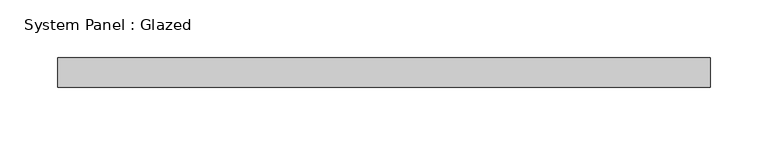
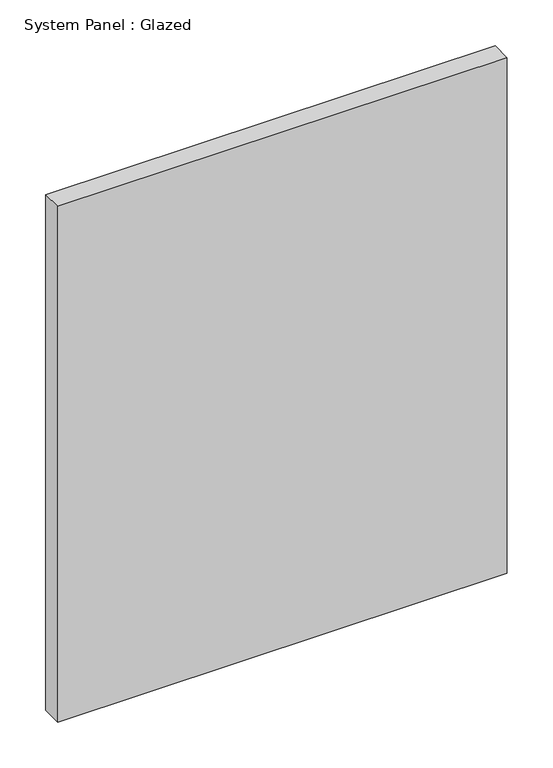
"""IFC4 building model written with IfcOpenShell, lengths in millimetres: plate geometry, System Panel : Glazed."""

from ifc_helpers import new_model, si_unit, origin, origin_with_axes, place, context, project, spatial, polyline, outline, extrude, source, transform, mapped, element, save


def system_panel_glazed_e7b2ff25(model_context):
    return source(origin(), model_context, "Body", "SweptSolid", [
        extrude(outline(polyline([(282.575, 19.05), (-282.575, 19.05), (-282.575, 44.45), (282.575, 44.45), (282.575, 19.05)])), origin_with_axes(), (0.0, 0.0, 1.0), 685.0309615),
    ])


if __name__ == "__main__":
    model = new_model("IFC4")
    model_context = context("Model", 3, world=origin())
    ifc_project = project(units=[si_unit("LENGTHUNIT", "METRE", prefix="MILLI")], contexts=[model_context])
    site = spatial("IfcSite", under=ifc_project)
    building = spatial("IfcBuilding", under=site)
    placement = place(None, origin())
    system_panel_glazed_shape = system_panel_glazed_e7b2ff25(model_context)
    element("IfcPlate", 1, ObjectType="System Panel : Glazed", at=placement, inside=building, context=model_context, shape_type="MappedRepresentation", body=[
        mapped(system_panel_glazed_shape, transform((0.0, 0.0, 0.0), x_axis=(1.0, 0.0, 0.0), y_axis=(0.0, 1.0, 0.0), z_axis=(0.0, 0.0, 1.0))),
    ])
    save(model, "model.ifc")

# Revit data of these elements
# Type "System Panel : Glazed"
#   Construction Type Id = "GSP4R"
#   Analytic Construction = "1/8 in Pilkington single glazing"
#   Visual Light Transmittance = 0.9
#   Solar Heat Gain Coefficient = 0.86
#   Heat Transfer Coefficient (U) = 1.18115 BTU/(h·ft²·°F)
#   Define Thermal Properties by = 1
# Element 1 (IfcPlate, "System Panel : Glazed")
#   Materials on its faces: "Glass"
# Materials
#   "Glass": class "Glass", colour RGB 0 128 192, transparency 0.75, Description = "Soda Lime Glass", Cost = 0
